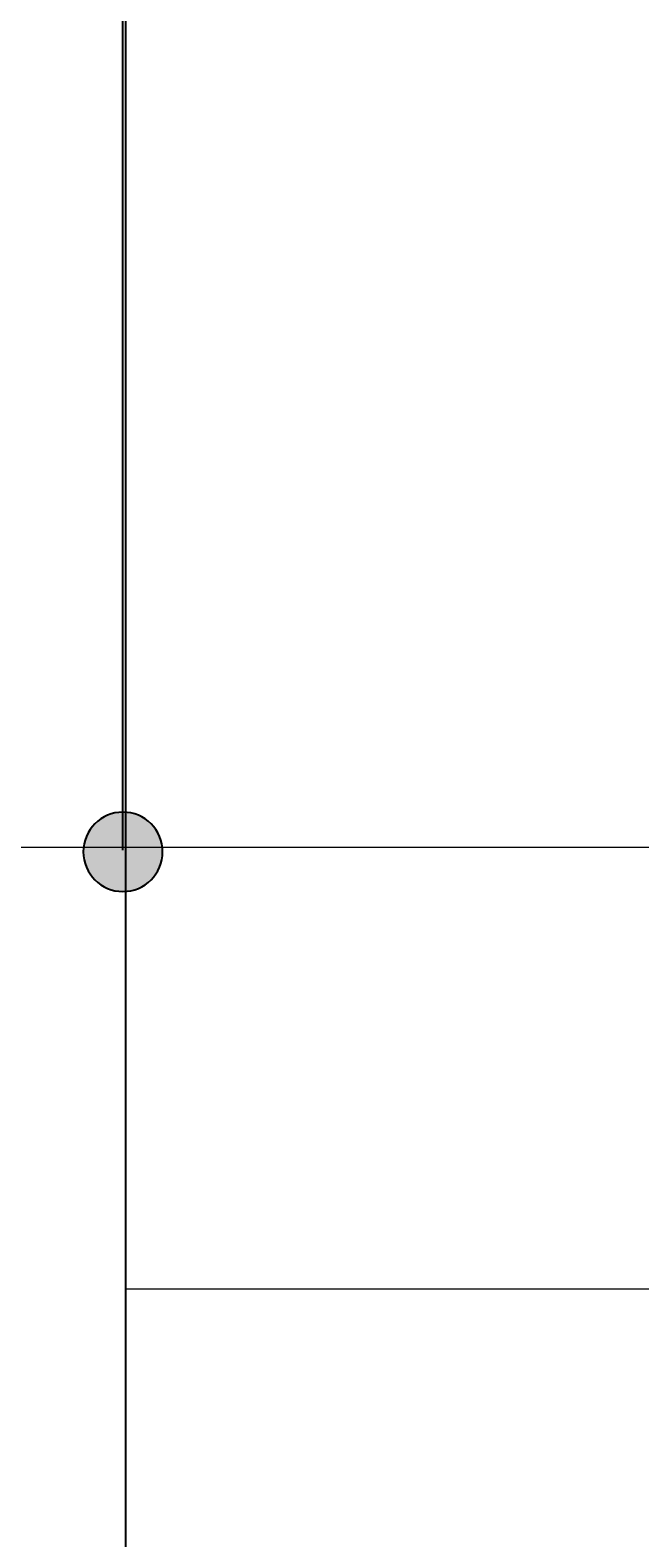
# Model space of a CAD drawing. Units: inches. Extents: x 738 to 1068, y 378 to 757.
# Tile 16 of 41: x 833 to 856, y 435 to 492. Entities that reach past the tile are written whole.
import ezdxf

# ---------------------------------------------------------------- set-up
doc = ezdxf.new("R2010")
doc.units = ezdxf.units.IN
doc.header["$MEASUREMENT"] = 0
for name, color, linetype, lineweight in [('A-ANNO-DIMS', 2, 'Continuous', 18), ('E-CONN', 7, 'Continuous', 25), ('E-CONN-PATT', 7, 'Continuous', 13), ('E-CTRL-WIRE', 7, 'Continuous', 18)]:
    doc.layers.add(name, color=color, linetype=linetype, lineweight=lineweight)
doc.styles.get("Standard").update_dxf_attribs({"font": 'arial.ttf'})
doc.dimstyles.get("Standard").update_dxf_attribs({"dimtxt": 0.18, "dimasz": 0.18, "dimexe": 0.18, "dimexo": 0.0625, "dimgap": 0.09, "dimtad": 0, "dimtih": 1, "dimtoh": 1, "dimdec": 4, "dimzin": 0, "dimdsep": 46, "dimtxsty": 'Standard', "dimcen": 0.09, "dimadec": 0, "dimazin": 0, "dimtfac": 1, "dimtdec": 4, "dimtofl": 0, "dimtmove": 0, "dimatfit": 3, "dimfxl": 1, "dimtolj": 1, "dimtzin": 0, "dimarcsym": 0})

# ---------------------------------------------------------------- blocks, each defined once
blk = doc.blocks.new('*D32')
at = {"layer": 'A-ANNO-DIMS', "color": 0, "lineweight": -2, "transparency": 16777216}
for p, q in [((809.38, 461.454), (809.38, 756.505)), ((809.56, 756.325), (822.41, 756.325)), ((836.052, 756.325), (823.202, 756.325)), ((836.232, 461.277), (836.232, 756.505))]:
    blk.add_line(p, q, dxfattribs=at)
at = {"layer": 'A-ANNO-DIMS', "color": 0, "transparency": 16777216}
for points in [[(809.56, 756.355), (809.56, 756.295), (809.38, 756.325)], [(836.052, 756.355), (836.052, 756.295), (836.232, 756.325)]]:
    blk.add_solid(points, dxfattribs=at)
at = {"layer": 'Defpoints', "color": 0, "transparency": 16777216}
for p in [(836.232, 756.325), (809.38, 461.392), (836.232, 461.214)]:
    blk.add_point(p, dxfattribs=at)
at = {"layer": 'A-ANNO-DIMS', "color": 0, "transparency": 16777216, "insert": (822.806, 756.325), "char_height": 0.18, "attachment_point": 5}
blk.add_mtext('\\A1;26.85', dxfattribs=at)
blk = doc.blocks.new('*D33')
at = {"layer": 'A-ANNO-DIMS', "color": 0, "lineweight": -2, "transparency": 16777216}
for p, q in [((836.324, 514.624), (836.324, 378.239)), ((907.171, 514.624), (907.171, 378.239)), ((836.504, 378.419), (871.354, 378.419)), ((906.991, 378.419), (872.141, 378.419))]:
    blk.add_line(p, q, dxfattribs=at)
at = {"layer": 'A-ANNO-DIMS', "color": 0, "transparency": 16777216}
for points in [[(836.504, 378.449), (836.504, 378.389), (836.324, 378.419)], [(906.991, 378.449), (906.991, 378.389), (907.171, 378.419)]]:
    blk.add_solid(points, dxfattribs=at)
at = {"layer": 'Defpoints', "color": 0, "transparency": 16777216}
for p in [(836.324, 514.687), (907.171, 514.687), (907.171, 378.419)]:
    blk.add_point(p, dxfattribs=at)
at = {"layer": 'A-ANNO-DIMS', "color": 0, "transparency": 16777216, "insert": (871.748, 378.419), "char_height": 0.18, "attachment_point": 5}
blk.add_mtext('\\A1;70.85', dxfattribs=at)
blk = doc.blocks.new('*D38')
at = {"layer": 'A-ANNO-DIMS', "color": 0, "lineweight": -2, "transparency": 16777216}
for p, q in [((781.485, 593.017), (781.485, 378.239)), ((887.04, 593.067), (887.04, 378.239)), ((781.665, 378.419), (833.807, 378.419)), ((886.86, 378.419), (834.718, 378.419))]:
    blk.add_line(p, q, dxfattribs=at)
at = {"layer": 'A-ANNO-DIMS', "color": 0, "transparency": 16777216}
for points in [[(781.665, 378.449), (781.665, 378.389), (781.485, 378.419)], [(886.86, 378.449), (886.86, 378.389), (887.04, 378.419)]]:
    blk.add_solid(points, dxfattribs=at)
at = {"layer": 'Defpoints', "color": 0, "transparency": 16777216}
for p in [(781.485, 593.08), (887.04, 593.13), (887.04, 378.419)]:
    blk.add_point(p, dxfattribs=at)
at = {"layer": 'A-ANNO-DIMS', "color": 0, "transparency": 16777216, "insert": (834.263, 378.419), "char_height": 0.18, "attachment_point": 5}
blk.add_mtext('\\A1;105.56', dxfattribs=at)

msp = doc.modelspace()

# ---------------------------------------------------------------- hatches: boundary and pattern name
at = {"layer": 'E-CONN-PATT'}
h = msp.add_hatch(color=256, dxfattribs=at)
h.dxf.hatch_style = 1
h.paths.add_polyline_path([(834.743, 461.3919), (837.7218, 461.3919, 0.8876841)])
h.paths.add_polyline_path([(837.7324, 461.214, 0.0297234), (837.7218, 461.3919), (834.743, 461.3919, 0.0297234), (834.7324, 461.214, 1)])
h.paths.add_polyline_path([(908.7522, 461.214, 0.0297234), (908.7416, 461.3919), (905.7628, 461.3919, 0.0297234), (905.7522, 461.214, 1)])
h.paths.add_polyline_path([(905.7628, 461.3919), (908.7416, 461.3919, 0.8876841)])

# ---------------------------------------------------------------- linework, layer by layer
at = {"layer": 'E-CONN'}
msp.add_lwpolyline([(834.7324, 461.214, 1), (837.7324, 461.214, 1)], format="xyb", close=True, dxfattribs=at)
at = {"layer": 'E-CTRL-WIRE'}
for p, q in [((809.3803, 461.3919), (865.0964, 461.3919)), ((836.3244, 444.6775), (836.3244, 459.6489)), ((866.3244, 444.6775), (836.3244, 444.6775))]:
    msp.add_line(p, q, dxfattribs=at)

# ---------------------------------------------------------------- dimensions: what is measured, and where the dimension line sits
at = {"layer": 'A-ANNO-DIMS'}
for base, p1, p2, picture, middle in [((836.2324, 756.3251), (809.3803, 461.3919), (836.2324, 461.214), '*D32', (822.8064, 756.3251)), ((887.0404, 378.4191), (781.4846, 593.0796), (887.0404, 593.1296), '*D38', (834.2625, 378.4191)), ((907.1708, 378.4191), (836.3244, 514.6866), (907.1708, 514.6866), '*D33', (871.7476, 378.4191))]:
    dim = msp.add_linear_dim(base=base, p1=p1, p2=p2, dimstyle='Standard', override={"dimdec": 2, "dimlfac": 1, "dimrnd": 0, "dimzin": 0, "dimdsep": 46, "dimlunit": 2}, dxfattribs=at)
    dim.commit()
    dim.dimension.update_dxf_attribs({"geometry": picture, "text_midpoint": middle})

doc.saveas('drawing.dxf')
